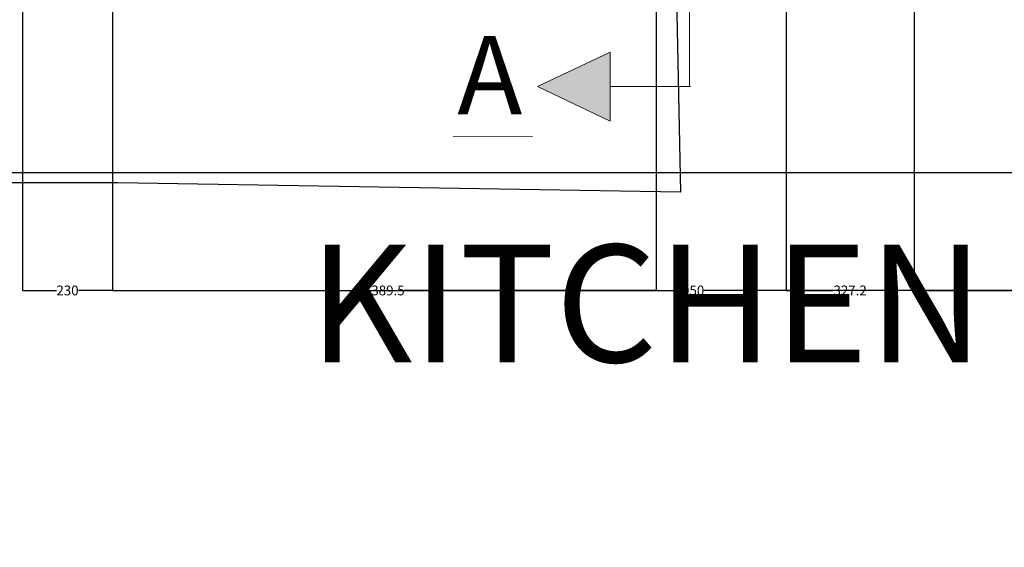
# Model space of a CAD drawing. Units: millimetres. Extents: x 1944 to 29915, y -10550 to 5909.
# Tile 3 of 24: x 6709 to 9226, y -1353 to -5. Entities that reach past the tile are written whole.
import ezdxf
from ezdxf import colors
from ezdxf.entities.mleader import LeaderData, LeaderLine
from ezdxf.math import Vec2, Vec3

# ---------------------------------------------------------------- set-up
doc = ezdxf.new("R2010")
doc.units = ezdxf.units.MM
doc.header["$MEASUREMENT"] = 0
for name, color, linetype, lineweight in [('A-ANNO-DIMS', 2, 'Continuous', 18), ('A-ANNO-SYMB', 2, 'Continuous', 18), ('A-ANNO-TEXT', 7, 'Continuous', 25), ('A-FLOR-FIXT', 9, 'Continuous', 18)]:
    doc.layers.add(name, color=color, linetype=linetype, lineweight=lineweight)
doc.styles.get("Standard").update_dxf_attribs({"font": 'arial.ttf'})
doc.dimstyles.get("Standard").update_dxf_attribs({"dimtxt": 25, "dimasz": 0.18, "dimexe": 0.18, "dimexo": 0.0625, "dimgap": 0.09, "dimtad": 0, "dimtih": 1, "dimtoh": 1, "dimdec": 0, "dimzin": 0, "dimdsep": 46, "dimtxsty": 'Standard', "dimcen": 0.09, "dimadec": 0, "dimazin": 0, "dimtfac": 1, "dimtdec": 0, "dimtofl": 0, "dimtmove": 0, "dimatfit": 3, "dimfxl": 1, "dimtolj": 1, "dimtzin": 0, "dimarcsym": 0})

# ---------------------------------------------------------------- blocks, each defined once
blk = doc.blocks.new('*D49')
at = {"layer": 'A-ANNO-DIMS', "color": 0, "lineweight": -2, "transparency": 16777216}
for p, q in [((8335.5, 4760.8), (8335.5, -697.2)), ((6945.9, 4530.8), (6945.9, -697.2)), ((6946.1, -697), (7589.8, -697)), ((8335.3, -697), (7691.6, -697))]:
    blk.add_line(p, q, dxfattribs=at)
at = {"layer": 'A-ANNO-DIMS', "color": 0, "transparency": 16777216}
for points in [[(6946.1, -697), (6946.1, -697.1), (6945.9, -697)], [(8335.3, -697), (8335.3, -697.1), (8335.5, -697)]]:
    blk.add_solid(points, dxfattribs=at)
at = {"layer": 'Defpoints', "color": 0, "transparency": 16777216}
for p in [(8335.5, 4760.8), (6945.9, 4530.8), (8335.5, -697)]:
    blk.add_point(p, dxfattribs=at)
at = {"layer": 'A-ANNO-DIMS', "color": 0, "transparency": 16777216, "insert": (7640.7, -697), "char_height": 25, "attachment_point": 5}
blk.add_mtext('\\A1;1389.5', dxfattribs=at)
blk = doc.blocks.new('*D50')
at = {"layer": 'A-ANNO-DIMS', "color": 0, "lineweight": -2, "transparency": 16777216}
for p, q in [((8995.2, 30.8), (8995.2, -697.2)), ((9895.2, 30.8), (9895.2, -697.2)), ((8995.4, -697), (9417.6, -697)), ((9895, -697), (9472.9, -697))]:
    blk.add_line(p, q, dxfattribs=at)
at = {"layer": 'A-ANNO-DIMS', "color": 0, "transparency": 16777216}
for points in [[(8995.4, -697), (8995.4, -697.1), (8995.2, -697)], [(9895, -697), (9895, -697.1), (9895.2, -697)]]:
    blk.add_solid(points, dxfattribs=at)
at = {"layer": 'Defpoints', "color": 0, "transparency": 16777216}
for p in [(8995.2, 30.8), (9895.2, 30.8), (9895.2, -697)]:
    blk.add_point(p, dxfattribs=at)
at = {"layer": 'A-ANNO-DIMS', "color": 0, "transparency": 16777216, "insert": (9445.2, -697), "char_height": 25, "attachment_point": 5}
blk.add_mtext('\\A1;900', dxfattribs=at)
blk = doc.blocks.new('*D52')
at = {"layer": 'A-ANNO-DIMS', "color": 0, "lineweight": -2, "transparency": 16777216}
for p, q in [((6715.9, 490.8), (6715.9, -697.2)), ((6945.9, 490.8), (6945.9, -697.2)), ((6716.1, -697), (6803.1, -697)), ((6945.8, -697), (6858.8, -697))]:
    blk.add_line(p, q, dxfattribs=at)
at = {"layer": 'A-ANNO-DIMS', "color": 0, "transparency": 16777216}
for points in [[(6716.1, -697), (6716.1, -697.1), (6715.9, -697)], [(6945.8, -697), (6945.8, -697.1), (6945.9, -697)]]:
    blk.add_solid(points, dxfattribs=at)
at = {"layer": 'Defpoints', "color": 0, "transparency": 16777216}
for p in [(6715.9, 490.8), (6945.9, 490.8), (6945.9, -697)]:
    blk.add_point(p, dxfattribs=at)
at = {"layer": 'A-ANNO-DIMS', "color": 0, "transparency": 16777216, "insert": (6830.9, -697), "char_height": 25, "attachment_point": 5}
blk.add_mtext('\\A1;230', dxfattribs=at)
blk = doc.blocks.new('*D53')
at = {"layer": 'A-ANNO-DIMS', "color": 0, "lineweight": -2, "transparency": 16777216}
for p, q in [((6945.94205, 490.774608), (6945.94205, -697.212556)), ((9895.94205, 490.774608), (9895.94205, -697.212556)), ((6946.12205, -697.032556), (8383.35205, -697.032556)), ((9895.76205, -697.032556), (8458.53205, -697.032556))]:
    blk.add_line(p, q, dxfattribs=at)
at = {"layer": 'A-ANNO-DIMS', "color": 0, "transparency": 16777216}
for points in [[(6946.12205, -697.002556), (6946.12205, -697.062556), (6945.94205, -697.032556)], [(9895.76205, -697.002556), (9895.76205, -697.062556), (9895.94205, -697.032556)]]:
    blk.add_solid(points, dxfattribs=at)
at = {"layer": 'Defpoints', "color": 0, "transparency": 16777216}
for p in [(6945.94205, 490.837108), (9895.94205, 490.837108), (9895.94205, -697.032556)]:
    blk.add_point(p, dxfattribs=at)
at = {"layer": 'A-ANNO-DIMS', "color": 0, "transparency": 16777216, "insert": (8420.94205, -697.032556), "char_height": 25, "attachment_point": 5}
blk.add_mtext('\\A1;2950', dxfattribs=at)
blk = doc.blocks.new('*D59')
at = {"layer": 'A-ANNO-DIMS', "color": 0, "lineweight": -2, "transparency": 16777216}
for p, q in [((8668, 4019.6), (8668, -697.2)), ((8995.2, 3870.8), (8995.2, -697.2)), ((8668.2, -697), (8789.5, -697)), ((8995, -697), (8873.8, -697))]:
    blk.add_line(p, q, dxfattribs=at)
at = {"layer": 'A-ANNO-DIMS', "color": 0, "transparency": 16777216}
for points in [[(8668.2, -697), (8668.2, -697.1), (8668, -697)], [(8995, -697), (8995, -697.1), (8995.2, -697)]]:
    blk.add_solid(points, dxfattribs=at)
at = {"layer": 'Defpoints', "color": 0, "transparency": 16777216}
for p in [(8668, 4019.6), (8995.2, 3870.8), (8995.2, -697)]:
    blk.add_point(p, dxfattribs=at)
at = {"layer": 'A-ANNO-DIMS', "color": 0, "transparency": 16777216, "insert": (8831.6, -697), "char_height": 25, "attachment_point": 5}
blk.add_mtext('\\A1;327.2', dxfattribs=at)
blk = doc.blocks.new('*D85')
at = {"layer": 'A-ANNO-DIMS', "color": 0, "lineweight": -2, "transparency": 16777216}
for p, q in [((6418.3, -1730.7), (6418.3, -395.6)), ((6418.5, -395.8), (15860.3, -395.8)), ((25389.1, -395.8), (15947.3, -395.8)), ((25389.3, -1846.5), (25389.3, -395.6))]:
    blk.add_line(p, q, dxfattribs=at)
at = {"layer": 'A-ANNO-DIMS', "color": 0, "transparency": 16777216}
for points in [[(6418.5, -395.7), (6418.5, -395.8), (6418.3, -395.8)], [(25389.1, -395.7), (25389.1, -395.8), (25389.3, -395.8)]]:
    blk.add_solid(points, dxfattribs=at)
at = {"layer": 'Defpoints', "color": 0, "transparency": 16777216}
for p in [(25389.3, -395.8), (6418.3, -1730.8), (25389.3, -1846.5)]:
    blk.add_point(p, dxfattribs=at)
at = {"layer": 'A-ANNO-DIMS', "color": 0, "transparency": 16777216, "insert": (15903.8, -395.8), "char_height": 25, "attachment_point": 5}
blk.add_mtext('\\A1;18971', dxfattribs=at)

msp = doc.modelspace()

# ---------------------------------------------------------------- hatches: boundary and pattern name
at = {"layer": 'A-ANNO-SYMB'}
h = msp.add_hatch(color=256, dxfattribs=at)
h.dxf.hatch_style = 1
h.paths.add_polyline_path([(8218.086, -88.239), (8032.549, -176.269), (8218.086, -264.3), (8218.086, -176.269)])

# ---------------------------------------------------------------- linework, layer by layer
for p, q in [((8420.942, -176.269), (8420.942, 5412.489)), ((7816.893, -304.783), (8019.494, -303.764))]:
    msp.add_line(p, q, dxfattribs=at)
at = {"layer": 'A-FLOR-FIXT'}
for p, q in [((8218.086, -88.239), (8032.549, -176.269)), ((8218.086, -176.269), (8218.086, -88.239)), ((8218.086, -264.3), (8032.549, -176.269)), ((8423.671, -176.269), (8218.086, -176.269)), ((8218.086, -176.269), (8218.086, -264.3))]:
    msp.add_line(p, q, dxfattribs=at)

# ---------------------------------------------------------------- texts
at = {"layer": 'A-ANNO-TEXT'}
for s, height, p in [('A', 200, (7827.54, -246.725)), ('KITCHEN PLAN ', 300, (7448.016, -880.236))]:
    msp.add_text(s, height=height, dxfattribs=at).set_placement(p)

# ---------------------------------------------------------------- dimensions: what is measured, and where the dimension line sits
at = {"layer": 'A-ANNO-DIMS'}
for base, p1, p2, override, picture, middle in [((8335.477, -697.033), (6945.942, 4530.837), (8335.477, 4760.837), {"dimdec": 1, "dimlfac": 1, "dimrnd": 0, "dimzin": 0, "dimdsep": 46, "dimlunit": 2}, '*D49', (7640.71, -697.033)), ((8995.217, -697.033), (8668.038, 4019.643), (8995.217, 3870.837), {"dimdec": 1, "dimlfac": 1, "dimrnd": 0, "dimzin": 0, "dimdsep": 46, "dimlunit": 2}, '*D59', (8831.628, -697.033)), ((6945.942, -697.033), (6715.942, 490.837), (6945.942, 490.837), {"dimdec": 0, "dimlfac": 1, "dimrnd": 0, "dimzin": 0, "dimdsep": 46, "dimlunit": 2}, '*D52', (6830.942, -697.033)), ((9895.942, -697.033), (6945.942, 490.837), (9895.942, 490.837), {"dimdec": 0, "dimlfac": 1, "dimrnd": 0, "dimzin": 0, "dimdsep": 46, "dimlunit": 2}, '*D53', (8420.942, -697.033)), ((9895.217, -697.033), (8995.217, 30.837), (9895.217, 30.837), {"dimdec": 0, "dimlfac": 1, "dimrnd": 0, "dimzin": 0, "dimdsep": 46, "dimlunit": 2}, '*D50', (9445.217, -697.033)), ((25389.297, -395.752), (6418.315, -1730.752), (25389.297, -1846.542), {"dimdec": 0, "dimlfac": 1, "dimrnd": 0, "dimzin": 0, "dimdsep": 46, "dimlunit": 2}, '*D85', (15903.806, -395.752))]:
    dim = msp.add_linear_dim(base=base, p1=p1, p2=p2, dimstyle='Standard', override=override, dxfattribs=at)
    dim.commit()
    dim.dimension.update_dxf_attribs({"geometry": picture, "text_midpoint": middle})

# ---------------------------------------------------------------- leaders
at = {"layer": 'A-ANNO-TEXT'}
ml = msp.add_multileader_mtext('Standard', dxfattribs=at)
ml.set_content('15 AMP POWER POINT \\PFOR MIXER', color=256)
ml.set_leader_properties()
ml.build(insert=Vec2(0, 0))
ml.multileader.update_dxf_attribs({"dogleg_length": 568.936, "arrow_head_size": 100})
ctx = ml.context
ctx.base_point, ctx.char_height, ctx.arrow_head_size, ctx.landing_gap_size, ctx.plane_origin = Vec3(4878.252, -422.117), 100, 100, 0.09, Vec3(6870.097, -798.764)
ctx.text_align_type = 2
notes = []
notes.append((ctx, [(0, (1, 1, 0), (6958.555, -422.117), (-1, 0), 568.936, [(0, [(8384.052, 260.837), (8397.606, -446.246)], 0, [])])]))
ctx.mtext.insert, ctx.mtext.alignment, ctx.mtext.flow_direction = Vec3(6389.529, -371.264), 3, 5
for ctx, leaders in notes:
    for number, flags, end, landing, length, lines in leaders:
        leader = LeaderData()
        leader.index, (leader.has_last_leader_line, leader.has_dogleg_vector, leader.attachment_direction) = number, flags
        leader.last_leader_point, leader.dogleg_vector, leader.dogleg_length = Vec3(end), Vec3(landing), length
        for number, points, colour, breaks in lines:
            line = LeaderLine()
            line.index, line.vertices, line.color, line.breaks = number, Vec3.list(points), colors.encode_raw_color(colour), breaks
            leader.lines.append(line)
        ctx.leaders.append(leader)

doc.saveas('drawing.dxf')
